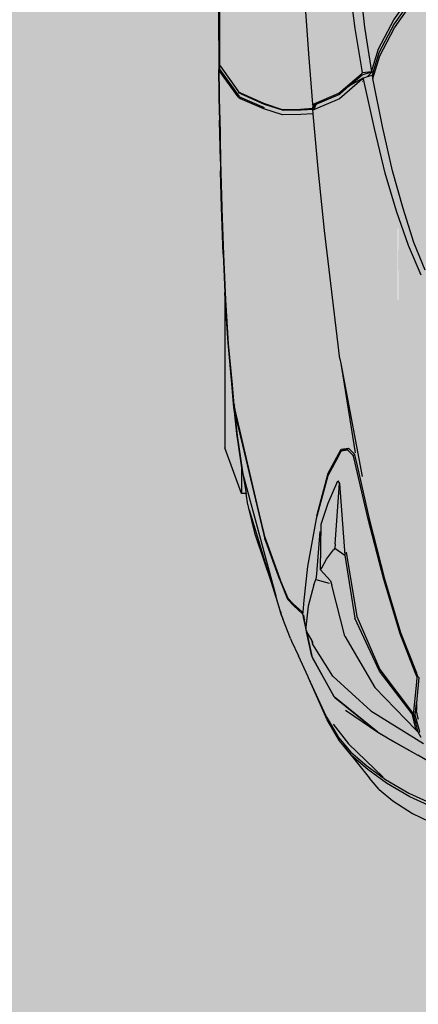
# Model space of a CAD drawing. Units: inches. Extents: x 1884 to 2398, y 474 to 1488.
# Tile 4 of 39: x 2186 to 2203, y 577 to 620. Entities that reach past the tile are written whole.
import ezdxf

# ---------------------------------------------------------------- set-up
doc = ezdxf.new("R2010")
doc.units = ezdxf.units.IN
doc.header["$MEASUREMENT"] = 0
doc.layers.get('0').update_dxf_attribs({"color": 250})
doc.layers.add('C-VEHI', color=8, linetype='Continuous', lineweight=18)
doc.layers.add('Edges', color=250, linetype='Continuous')
doc.layers.add('L-PVMT-PATT', color=9, linetype='Continuous', lineweight=13, true_color=0xc7c8ca)

# ---------------------------------------------------------------- blocks, each defined once
blk = doc.blocks.new('Nissan Qashqai pl')
at = {"layer": 'Edges'}
for p, q in [((11.4732, 11.2592), (11.4658, 11.2461)), ((11.5074, 11.2362), (11.5165, 11.256)), ((11.5206, 11.2572), (11.5113, 11.2372)), ((11.5295, 11.24), (11.5384, 11.2583)), ((10.6583, 11.2197), (10.6215, 11.2456)), ((10.6261, 11.2458), (10.6627, 11.22)), ((10.6671, 11.2203), (10.6306, 11.2459)), ((10.933, 11.2541), (10.9026, 11.2417)), ((10.9384, 11.2497), (10.9059, 11.2355)), ((11.3311, 11.227), (11.3751, 11.2443)), ((11.38, 11.2453), (11.3747, 11.2431)), ((11.3751, 11.2443), (11.3752, 11.2444)), ((11.3751, 11.2443), (11.3762, 11.2443)), ((11.3792, 11.2459), (11.3752, 11.2444)), ((11.3763, 11.2444), (11.3752, 11.2444)), ((11.3792, 11.2459), (11.3804, 11.2469)), ((11.3793, 11.2463), (11.3792, 11.2459)), ((11.3853, 11.2449), (11.38, 11.2453)), ((11.3804, 11.2469), (11.4082, 11.2444)), ((11.4212, 11.2412), (11.3853, 11.2449)), ((11.3915, 11.1988), (11.4381, 11.244)), ((11.4164, 11.2444), (11.4082, 11.2444)), ((11.409, 11.2443), (11.4082, 11.2444)), ((11.409, 11.2443), (11.4163, 11.2443)), ((11.4152, 11.2437), (11.409, 11.2443)), ((11.4163, 11.2443), (11.4152, 11.2437)), ((11.4215, 11.2431), (11.4152, 11.2437)), ((11.4164, 11.2444), (11.4163, 11.2443)), ((11.4169, 11.2446), (11.4164, 11.2444)), ((11.4252, 11.2462), (11.4169, 11.2446)), ((11.417, 11.1942), (11.4529, 11.252)), ((11.4315, 11.244), (11.4229, 11.2416)), ((11.44, 11.2482), (11.423, 11.2435)), ((11.4266, 11.2465), (11.4252, 11.2462)), ((11.4381, 11.244), (11.4292, 11.2418)), ((11.4403, 11.2464), (11.4315, 11.244)), ((11.4381, 11.244), (11.4403, 11.2464)), ((11.4403, 11.2464), (11.44, 11.2482)), ((11.4462, 11.2495), (11.4403, 11.2464)), ((11.4411, 11.2028), (11.4656, 11.2458)), ((11.447, 11.2127), (11.4656, 11.2458)), ((11.4656, 11.2458), (11.4658, 11.2461)), ((10.9026, 11.2417), (10.8653, 11.2297)), ((10.9059, 11.2355), (10.8682, 11.2226)), ((11.3747, 11.2431), (11.3323, 11.2264)), ((11.3715, 11.2043), (11.4177, 11.2389)), ((11.4203, 11.2398), (11.3733, 11.2037)), ((11.4177, 11.2389), (11.4193, 11.24)), ((11.4192, 11.2397), (11.4194, 11.24)), ((11.4193, 11.24), (11.4196, 11.2402)), ((11.4194, 11.24), (11.4193, 11.24)), ((11.4194, 11.24), (11.4196, 11.2402)), ((11.4196, 11.2399), (11.4194, 11.24)), ((11.4196, 11.2402), (11.4201, 11.2405)), ((11.4198, 11.2401), (11.4201, 11.2405)), ((11.4201, 11.2405), (11.4212, 11.2412)), ((11.4292, 11.2418), (11.4203, 11.2398)), ((11.4229, 11.2416), (11.4203, 11.2398)), ((11.4212, 11.2412), (11.4215, 11.2431)), ((11.4218, 11.2413), (11.4212, 11.2412)), ((11.423, 11.2435), (11.4215, 11.2431)), ((11.4229, 11.2416), (11.4218, 11.2413)), ((11.4222, 11.2413), (11.4218, 11.2413)), ((11.423, 11.2435), (11.4229, 11.2416)), ((11.4924, 11.2103), (11.5074, 11.2362)), ((11.5113, 11.2372), (11.4963, 11.2114)), ((11.5158, 11.2186), (11.5295, 11.24)), ((10.8653, 11.2297), (10.8239, 11.2181)), ((10.8682, 11.2226), (10.8264, 11.21)), ((11.272, 11.2092), (11.3311, 11.227)), ((11.3323, 11.2264), (11.2728, 11.2084)), ((10.69, 11.2028), (10.6583, 11.2197)), ((10.6627, 11.22), (10.6943, 11.2032)), ((10.6976, 11.2041), (10.6671, 11.2203)), ((10.8239, 11.2181), (10.7754, 11.2071)), ((11.447, 11.2127), (11.4411, 11.2028)), ((11.4963, 11.2114), (11.4815, 11.191)), ((11.5033, 11.2034), (11.5158, 11.2186)), ((10.7155, 11.1952), (10.69, 11.2028)), ((10.6943, 11.2032), (10.7155, 11.1969)), ((10.7228, 11.1965), (10.6976, 11.2041)), ((10.7754, 11.2071), (10.7228, 11.1965)), ((10.8264, 11.21), (10.7776, 11.1982)), ((11.2063, 11.1926), (11.272, 11.2092)), ((11.2728, 11.2084), (11.2066, 11.1914)), ((11.3132, 11.1789), (11.3715, 11.2043)), ((11.3733, 11.2037), (11.3153, 11.1769)), ((11.4405, 11.2018), (11.4014, 11.1541)), ((11.4022, 11.1548), (11.4405, 11.2018)), ((11.4163, 11.1666), (11.4405, 11.2018)), ((11.4408, 11.2022), (11.4405, 11.2018)), ((11.4411, 11.2028), (11.4408, 11.2022)), ((11.4411, 11.2028), (11.4411, 11.2028)), ((11.4531, 11.1697), (11.4897, 11.2077)), ((11.4774, 11.1898), (11.4924, 11.2103)), ((11.5033, 11.2034), (11.4936, 11.195)), ((10.6664, 11.1875), (10.7155, 11.1952)), ((10.7155, 11.1957), (10.7155, 11.1969)), ((10.7155, 11.1969), (10.7192, 11.1957)), ((10.7209, 11.1902), (10.7155, 11.1957)), ((10.7155, 11.1952), (10.7155, 11.1957)), ((10.7186, 11.1848), (10.7155, 11.1952)), ((10.7155, 11.1952), (10.7165, 11.1851)), ((10.7192, 11.1957), (10.7228, 11.1965)), ((10.7192, 11.1957), (10.7209, 11.1902)), ((10.7209, 11.1902), (10.7221, 11.1861)), ((10.7776, 11.1982), (10.7247, 11.1867)), ((11.2066, 11.1914), (11.1401, 11.1759)), ((11.148, 11.1791), (11.2063, 11.1926)), ((11.335, 11.1656), (11.3915, 11.1988)), ((11.379, 11.1527), (11.417, 11.1942)), ((11.4543, 11.1636), (11.4908, 11.1928)), ((11.4624, 11.1725), (11.4774, 11.1898)), ((11.4815, 11.191), (11.4662, 11.1736)), ((11.4936, 11.195), (11.4908, 11.1928)), ((10.6144, 11.1813), (10.6664, 11.1875)), ((10.7137, 11.1846), (10.6678, 11.177)), ((10.7165, 11.1851), (10.7137, 11.1846)), ((10.7177, 11.1838), (10.7165, 11.1851)), ((10.7387, 11.1593), (10.7177, 11.1838)), ((10.7312, 11.1701), (10.7186, 11.1848)), ((10.7221, 11.1861), (10.7222, 11.1859)), ((10.7222, 11.186), (10.7221, 11.1861)), ((10.7247, 11.1867), (10.7222, 11.186)), ((10.7222, 11.186), (10.7222, 11.1859)), ((10.7222, 11.1859), (10.7232, 11.1848)), ((10.7222, 11.1859), (10.7224, 11.1855)), ((10.7224, 11.1855), (10.7312, 11.1701)), ((10.7232, 11.1848), (10.7228, 11.1859)), ((10.7232, 11.1848), (10.7449, 11.1598)), ((10.7257, 11.1853), (10.7256, 11.1854)), ((11.0357, 11.1613), (11.1598, 11.1847)), ((11.1358, 11.1765), (11.148, 11.1791)), ((11.2428, 11.1673), (11.3132, 11.1789)), ((10.6678, 11.177), (10.6152, 11.1702)), ((10.7397, 11.1602), (10.7312, 11.1701)), ((11.0492, 11.1635), (11.1336, 11.1772)), ((11.1285, 11.1697), (11.1293, 11.1705)), ((11.1298, 11.1618), (11.1285, 11.1697)), ((11.1293, 11.1705), (11.1353, 11.1764)), ((11.1293, 11.1705), (11.1306, 11.163)), ((11.1347, 11.1731), (11.1306, 11.169)), ((11.1306, 11.169), (11.1319, 11.1614)), ((11.1366, 11.175), (11.1347, 11.1731)), ((11.1353, 11.1764), (11.1358, 11.1765)), ((11.1358, 11.1765), (11.1366, 11.175)), ((11.1401, 11.1759), (11.1366, 11.175)), ((11.2459, 11.1656), (11.3153, 11.1769)), ((11.4314, 11.1531), (11.4531, 11.1697)), ((11.4464, 11.1588), (11.4624, 11.1725)), ((11.4662, 11.1736), (11.4543, 11.1636)), ((10.7501, 11.1327), (10.7387, 11.1593)), ((10.7507, 11.1344), (10.7397, 11.1602)), ((10.7449, 11.1598), (10.7563, 11.1333)), ((11.0304, 11.1603), (10.8896, 11.1434)), ((11.0304, 11.1603), (11.0357, 11.1613)), ((11.0357, 11.1613), (11.0491, 11.1635)), ((11.0492, 11.1635), (11.0491, 11.1635)), ((11.156, 11.1476), (11.1298, 11.1618)), ((11.1319, 11.1614), (11.1306, 11.163)), ((11.1319, 11.1614), (11.1365, 11.159)), ((11.1365, 11.159), (11.1589, 11.147)), ((11.1644, 11.1579), (11.1672, 11.1598)), ((11.189, 11.1473), (11.1644, 11.1579)), ((11.1672, 11.1598), (11.2459, 11.1656)), ((11.2337, 11.155), (11.1672, 11.1598)), ((11.2382, 11.1549), (11.2459, 11.1656)), ((11.335, 11.1656), (11.2791, 11.1515)), ((11.4243, 11.1459), (11.4464, 11.1588)), ((11.4498, 11.1598), (11.4267, 11.1463)), ((11.4543, 11.1636), (11.4498, 11.1598)), ((11.2029, 11.1349), (11.156, 11.1476)), ((11.1589, 11.147), (11.2062, 11.1344)), ((11.2121, 11.1399), (11.189, 11.1473)), ((11.2337, 11.155), (11.2382, 11.1549)), ((11.2382, 11.1549), (11.2401, 11.1534)), ((11.2505, 11.1455), (11.2401, 11.1534)), ((11.2743, 11.1499), (11.2622, 11.139)), ((11.2729, 11.1338), (11.2766, 11.1485)), ((11.2743, 11.1499), (11.2791, 11.1515)), ((11.379, 11.1527), (11.3434, 11.1303)), ((11.4014, 11.1541), (11.3571, 11.1296)), ((11.3583, 11.13), (11.4014, 11.1541)), ((11.4267, 11.1463), (11.3807, 11.1259)), ((11.4022, 11.1548), (11.4014, 11.1541)), ((10.8218, 11.1365), (10.7615, 11.1311)), ((10.8896, 11.1434), (10.8218, 11.1365)), ((11.2622, 11.139), (11.2121, 11.1399)), ((11.2199, 11.1382), (11.2666, 11.1345)), ((11.2601, 11.1405), (11.2505, 11.1455)), ((11.2622, 11.139), (11.2601, 11.1405)), ((11.4228, 11.1453), (11.3807, 11.1259)), ((11.4228, 11.1453), (11.4243, 11.1459)), ((10.6318, 11.1213), (10.6955, 11.1257)), ((10.6955, 11.1257), (10.7509, 11.1302)), ((10.7507, 11.1309), (10.7501, 11.1327)), ((10.7511, 11.1335), (10.7507, 11.1344)), ((10.7507, 11.1344), (10.7524, 11.1335)), ((10.751, 11.131), (10.7507, 11.1309)), ((10.7509, 11.1302), (10.7507, 11.1309)), ((10.7522, 11.1311), (10.7509, 11.1302)), ((10.7516, 11.131), (10.7509, 11.1302)), ((10.7519, 11.1314), (10.7511, 11.1335)), ((10.7519, 11.1314), (10.7516, 11.131)), ((10.7522, 11.1311), (10.7516, 11.131)), ((10.7526, 11.1318), (10.7519, 11.1314)), ((10.7553, 11.1307), (10.7522, 11.1311)), ((10.7524, 11.1335), (10.7526, 11.1318)), ((10.7524, 11.1335), (10.7556, 11.1319)), ((10.7532, 11.1321), (10.7526, 11.1318)), ((10.7526, 11.1318), (10.7526, 11.1314)), ((10.7556, 11.1319), (10.7532, 11.1321)), ((10.7563, 11.1169), (10.7553, 11.1307)), ((10.7556, 11.1319), (10.7561, 11.1317)), ((10.7563, 11.1319), (10.7561, 11.1319)), ((10.7563, 11.1315), (10.7561, 11.1317)), ((10.7561, 11.1317), (10.7563, 11.1317)), ((10.7563, 11.1333), (10.7569, 11.1317)), ((10.7563, 11.1317), (10.7563, 11.1319)), ((10.7563, 11.1317), (10.7569, 11.1317)), ((10.7569, 11.1316), (10.7563, 11.1317)), ((10.7563, 11.1315), (10.7563, 11.1317)), ((10.7572, 11.1178), (10.7563, 11.1315)), ((10.7573, 11.1307), (10.7563, 11.1315)), ((10.7569, 11.1317), (10.7569, 11.1316)), ((10.7569, 11.1316), (10.7573, 11.1307)), ((10.7604, 11.131), (10.7573, 11.1307)), ((10.7615, 11.1311), (10.7604, 11.131)), ((10.7615, 11.1311), (10.7623, 11.1173)), ((11.2029, 11.1349), (11.2029, 11.1349)), ((11.2029, 11.1349), (11.2062, 11.1344)), ((11.2062, 11.1344), (11.2583, 11.1246)), ((11.2666, 11.1345), (11.2729, 11.1338)), ((11.2787, 11.1318), (11.2729, 11.1338)), ((11.2787, 11.1318), (11.3022, 11.1256)), ((11.3022, 11.1256), (11.3252, 11.1229)), ((11.3296, 11.1235), (11.3571, 11.1296)), ((11.3571, 11.1296), (11.3302, 11.1238)), ((11.3302, 11.1238), (11.3394, 11.129)), ((11.3394, 11.129), (11.342, 11.1305)), ((11.3394, 11.129), (11.3434, 11.1303)), ((11.3796, 11.1255), (11.3566, 11.1148)), ((11.3571, 11.1296), (11.3583, 11.13)), ((11.3807, 11.1259), (11.3796, 11.1255)), ((10.7565, 11.0969), (10.7563, 11.1169)), ((10.7575, 11.0979), (10.7572, 11.1178)), ((10.7623, 11.1173), (10.7626, 11.0974)), ((11.2583, 11.1246), (11.2956, 11.1208)), ((11.2956, 11.1208), (11.3085, 11.1195)), ((11.3, 11.1092), (11.3081, 11.1188)), ((11.3103, 11.1192), (11.3018, 11.1096)), ((11.308, 11.1188), (11.3086, 11.1195)), ((11.3081, 11.1188), (11.3086, 11.1195)), ((11.3085, 11.1195), (11.3086, 11.1195)), ((11.3086, 11.1195), (11.3103, 11.1193)), ((11.3103, 11.1193), (11.3103, 11.1192)), ((11.3103, 11.1193), (11.3106, 11.1193)), ((11.3106, 11.1193), (11.314, 11.1204)), ((11.317, 11.1214), (11.3119, 11.1206)), ((11.3132, 11.1199), (11.3259, 11.1227)), ((11.3242, 11.1226), (11.314, 11.1204)), ((11.314, 11.1204), (11.317, 11.1214)), ((11.3242, 11.1226), (11.317, 11.1214)), ((11.3198, 11.1231), (11.3252, 11.1229)), ((11.3242, 11.1226), (11.3259, 11.1227)), ((11.3252, 11.1229), (11.3283, 11.1228)), ((11.3259, 11.1227), (11.3283, 11.1228)), ((11.3283, 11.1228), (11.3296, 11.1235)), ((11.3296, 11.1235), (11.3302, 11.1238)), ((11.3405, 11.1072), (11.3566, 11.1148)), ((11.2946, 11.1033), (11.2736, 11.0947)), ((11.2741, 11.0952), (11.2934, 11.1031)), ((11.2934, 11.1031), (11.3, 11.1092)), ((11.3018, 11.1096), (11.2946, 11.1033)), ((11.3376, 11.106), (11.3161, 11.0975)), ((11.3376, 11.106), (11.3405, 11.1072)), ((10.7497, 11.0763), (10.7565, 11.0969)), ((10.7507, 11.0773), (10.7575, 11.0979)), ((10.7626, 11.0974), (10.7559, 11.0767)), ((11.2732, 11.0945), (11.2277, 11.0779)), ((11.2304, 11.0792), (11.2719, 11.0943)), ((11.2719, 11.0943), (11.2741, 11.0952)), ((11.2736, 11.0947), (11.2732, 11.0945)), ((11.2736, 11.0947), (11.2741, 11.0952)), ((11.2757, 11.085), (11.3124, 11.0963)), ((11.3124, 11.0963), (11.2907, 11.0899)), ((11.308, 11.0951), (11.3088, 11.0953)), ((11.3124, 11.0963), (11.3161, 11.0975)), ((11.1582, 11.0542), (11.2907, 11.0899)), ((11.1963, 11.0607), (11.2757, 11.085)), ((11.2247, 11.0677), (11.2757, 11.085)), ((10.7385, 11.051), (10.7497, 11.0763)), ((10.7396, 11.0519), (10.7507, 11.0773)), ((10.7549, 11.0776), (10.743, 11.0503)), ((10.7559, 11.0767), (10.7448, 11.0511)), ((11.0865, 11.045), (11.22, 11.0761)), ((11.2222, 11.0766), (11.0882, 11.045)), ((11.0918, 11.0453), (11.2222, 11.0766)), ((11.22, 11.0761), (11.2222, 11.0766)), ((11.2271, 11.0777), (11.2222, 11.0766)), ((11.2224, 11.0767), (11.2222, 11.0766)), ((11.2222, 11.0766), (11.2222, 11.0766)), ((11.2224, 11.0767), (11.2253, 11.0774)), ((11.2253, 11.0774), (11.2304, 11.0792)), ((11.2296, 11.0784), (11.2271, 11.0777)), ((11.2277, 11.0779), (11.2271, 11.0777)), ((11.2273, 11.0778), (11.2271, 11.0778)), ((11.2296, 11.0784), (11.2277, 11.0779)), ((11.193, 11.0596), (11.2215, 11.0666)), ((11.2215, 11.0666), (11.2247, 11.0677)), ((10.7424, 11.0499), (10.7125, 11.0285)), ((10.7363, 11.0483), (10.7376, 11.0492)), ((10.7387, 11.0502), (10.7376, 11.0492)), ((10.7376, 11.0492), (10.7378, 11.0495)), ((10.7378, 11.0495), (10.7385, 11.051)), ((10.7378, 11.0495), (10.7379, 11.0496)), ((10.7387, 11.0502), (10.7396, 11.0519)), ((10.7424, 11.0499), (10.743, 11.0503)), ((10.744, 11.0494), (10.7432, 11.0488)), ((10.7448, 11.0511), (10.744, 11.0494)), ((11.1475, 11.0521), (11.1123, 11.0472)), ((11.1147, 11.0476), (11.1547, 11.0532)), ((11.1783, 11.0521), (11.1283, 11.0341)), ((11.1525, 11.0528), (11.1475, 11.0521)), ((11.1475, 11.0521), (11.1783, 11.0521)), ((11.1547, 11.0532), (11.1525, 11.0528)), ((11.1547, 11.0532), (11.1783, 11.0572)), ((11.1906, 11.0592), (11.1783, 11.0572)), ((11.1783, 11.0572), (11.1783, 11.0521)), ((11.1909, 11.0593), (11.1906, 11.0592)), ((11.1909, 11.0593), (11.193, 11.0596)), ((10.7087, 11.0289), (10.7363, 11.0483)), ((10.7429, 11.0485), (10.7148, 11.0284)), ((10.7429, 11.0488), (10.7432, 11.0488)), ((10.7432, 11.0488), (10.7429, 11.0485)), ((11.0576, 11.0416), (11.0127, 11.0375)), ((11.0138, 11.0377), (11.059, 11.0419)), ((11.0798, 11.0434), (11.0576, 11.0416)), ((11.059, 11.0419), (11.0768, 11.0434)), ((11.0768, 11.0434), (11.0811, 11.0437)), ((11.087, 11.0442), (11.0798, 11.0434)), ((11.0811, 11.0444), (11.0821, 11.0442)), ((11.0811, 11.0437), (11.0827, 11.0441)), ((11.0827, 11.0441), (11.0856, 11.0448)), ((11.0827, 11.0441), (11.0836, 11.0439)), ((11.0882, 11.045), (11.0836, 11.0439)), ((11.0836, 11.0439), (11.087, 11.0442)), ((11.0856, 11.0448), (11.0865, 11.045)), ((11.0865, 11.045), (11.088, 11.0451)), ((11.087, 11.0442), (11.0872, 11.0442)), ((11.0873, 11.0443), (11.0872, 11.0442)), ((11.0873, 11.0443), (11.0883, 11.0444)), ((11.0883, 11.0444), (11.1147, 11.0476)), ((11.1123, 11.0472), (11.0883, 11.0444)), ((10.6151, 11.0283), (10.6644, 11.028)), ((10.6651, 11.0274), (10.6176, 11.0277)), ((10.6644, 11.028), (10.7078, 11.0282)), ((10.677, 11.0275), (10.6651, 11.0274)), ((10.7082, 11.0285), (10.6729, 11.0284)), ((10.68, 11.0274), (10.677, 11.0275)), ((10.6809, 11.0274), (10.68, 11.0274)), ((10.6809, 11.0274), (10.7128, 11.0275)), ((10.7078, 11.0282), (10.7083, 11.0285)), ((10.7082, 11.0285), (10.7078, 11.0282)), ((10.7085, 11.0289), (10.7082, 11.0285)), ((10.7083, 11.0285), (10.7082, 11.0285)), ((10.7083, 11.0285), (10.7087, 11.0289)), ((10.7125, 11.0285), (10.7083, 11.0285)), ((10.7146, 11.0286), (10.7125, 11.0285)), ((10.7125, 11.0285), (10.7139, 11.0278)), ((10.7134, 11.0275), (10.7128, 11.0275)), ((10.7625, 11.0281), (10.7134, 11.0275)), ((10.724, 11.0275), (10.7134, 11.0275)), ((10.7148, 11.0284), (10.7139, 11.0278)), ((10.7628, 11.0283), (10.7139, 11.0278)), ((10.724, 11.0275), (10.7685, 11.0281)), ((10.7628, 11.0281), (10.7625, 11.0281)), ((10.7628, 11.0283), (10.8131, 11.0292)), ((10.7628, 11.0281), (10.8131, 11.029)), ((10.7688, 11.0281), (10.7685, 11.0281)), ((10.8131, 11.029), (10.7688, 11.0281)), ((10.8131, 11.0292), (10.8644, 11.0306)), ((10.8132, 11.029), (10.8131, 11.029)), ((10.8132, 11.029), (10.8139, 11.029)), ((10.8142, 11.029), (10.8139, 11.029)), ((10.8142, 11.029), (10.8241, 11.0293)), ((10.8142, 11.029), (10.8142, 11.029)), ((10.8242, 11.0293), (10.8241, 11.0293)), ((10.8246, 11.0293), (10.8242, 11.0293)), ((10.8642, 11.0304), (10.8246, 11.0293)), ((10.9152, 11.0321), (10.8642, 11.0304)), ((10.8642, 11.0305), (10.8759, 11.031)), ((10.8644, 11.0306), (10.8759, 11.031)), ((10.8759, 11.031), (10.9158, 11.0324)), ((10.9152, 11.0321), (10.9577, 11.0341)), ((10.9158, 11.0324), (10.9657, 11.0347)), ((10.9649, 11.0344), (10.9577, 11.0341)), ((10.9577, 11.0341), (11.1283, 11.0341)), ((11.0127, 11.0375), (10.9649, 11.0344)), ((10.9657, 11.0347), (11.0138, 11.0377))]:
    blk.add_line(p, q, dxfattribs=at)
blk = doc.blocks.new('car')
blk.add_blockref('Nissan Qashqai pl', (-9.7433, -11.9151))
blk = doc.blocks.new('carr')
blk.add_blockref('car', (0.5124, -0.007))

msp = doc.modelspace()

# ---------------------------------------------------------------- hatches: boundary and pattern name
at = {"layer": 'L-PVMT-PATT'}
h = msp.add_hatch(color=256, dxfattribs=at)
h.dxf.hatch_style = 1
h.paths.add_polyline_path([(2387.529, 769.966), (2351.529, 769.966), (2238.447, 769.966), (2238.447, 762.15), (2238.447, 754.445), (2126.529, 754.445), (2126.529, 676.183), (2134.868, 676.183), (2142.673, 676.183), (2142.673, 646.578), (2134.868, 646.578), (2126.529, 646.578), (2126.529, 640.17), (2387.529, 640.17)])
h.paths.add_polyline_path([(2387.529, 631.385), (2303.086, 631.385), (2303.086, 615.671), (2387.529, 615.671)])
h.paths.add_polyline_path([(2387.529, 640.17), (2126.529, 640.17), (2126.529, 631.385), (2387.529, 631.385)])
h.paths.add_polyline_path([(2393.529, 604.13), (2387.529, 604.13), (2387.529, 615.671), (2303.086, 615.671), (2303.086, 607.943), (2249.649, 607.943), (2126.529, 607.943), (2126.529, 533.885), (2393.529, 533.885)])
h.paths.add_polyline_path([(2257.825, 611.008), (2257.83, 611.337), (2257.915, 616.493), (2258.021, 621.805), (2258.146, 627.274), (2258.252, 631.385), (2126.529, 631.385), (2126.529, 611.008)])
h.paths.add_polyline_path([(2258.892, 611.285), (2258.888, 611.008), (2300.247, 611.008), (2300.247, 631.385), (2259.314, 631.385), (2259.206, 627.173), (2259.081, 621.72), (2258.976, 616.424)])
h = msp.add_hatch(color=256, dxfattribs=at)
h.dxf.hatch_style = 1
h.paths.add_polyline_path([(2202.48, 609.653), (2202.489, 611.008), (2126.529, 611.008), (2126.529, 607.943), (2202.484, 607.943), (2202.48, 609.055), (2202.481, 609.184)])
h.paths.add_polyline_path([(2210.813, 611.008), (2208.615, 611.008), (2208.784, 609.602), (2209.041, 607.943), (2209.165, 607.943), (2209.383, 608.672), (2210.05, 609.923)])
h.paths.add_polyline_path([(2208.179, 611.008), (2206.175, 611.008), (2206.177, 610.963), (2206.351, 608.458), (2206.392, 607.943), (2208.635, 607.943), (2208.367, 609.547)])
h.paths.add_polyline_path([(2206.177, 610.963), (2206.175, 611.008), (2204.958, 611.008), (2204.951, 610.183), (2204.925, 610.11), (2204.493, 610.081), (2204.129, 610.077), (2204.054, 610.147), (2203.949, 611.008), (2202.51, 611.008), (2202.503, 609.679), (2202.511, 607.972), (2202.537, 607.943), (2206.392, 607.943), (2206.351, 608.458)])
h.paths.add_polyline_path([(2204.425, 611.008), (2203.949, 611.008), (2204.054, 610.147), (2204.489, 610.176)], flags=17)
h.paths.add_polyline_path([(2204.958, 611.008), (2204.517, 611.008), (2204.581, 610.179), (2204.951, 610.183)], flags=17)
h.paths.add_polyline_path([(2204.517, 611.008), (2204.425, 611.008), (2204.489, 610.176), (2204.581, 610.179)], flags=17)
h.paths.add_polyline_path([(2204.489, 610.176), (2204.054, 610.147), (2204.129, 610.077), (2204.485, 610.101), (2204.561, 610.106)], flags=17)
h.paths.add_polyline_path([(2204.581, 610.179), (2204.489, 610.176), (2204.561, 610.106)], flags=17)
h.paths.add_polyline_path([(2204.951, 610.183), (2204.581, 610.179), (2204.561, 610.106), (2204.925, 610.11)], flags=17)
h.paths.add_polyline_path([(2204.925, 610.11), (2204.561, 610.106), (2204.485, 610.101), (2204.493, 610.081)], flags=17)
h.paths.add_polyline_path([(2204.485, 610.101), (2204.129, 610.077), (2204.493, 610.081)], flags=16)

# ---------------------------------------------------------------- block references
at = {"layer": 'C-VEHI', "xscale": 39.37007874015748, "yscale": 39.37007874015748, "zscale": 39.37007874015748, "rotation": 270}
msp.add_blockref('carr', (2229.977, 676.232), dxfattribs=at)

doc.saveas('drawing.dxf')
